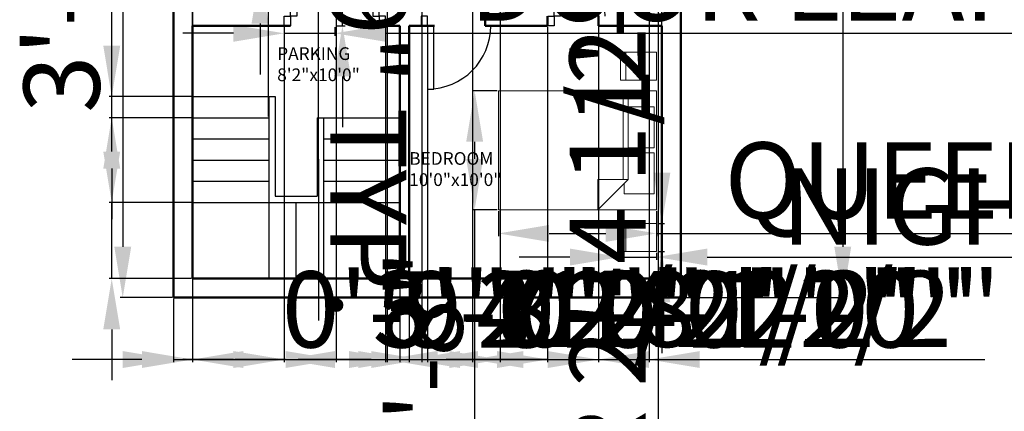
# Model space of a CAD drawing. Units: inches. Extents: x 1102 to 2414, y 295 to 1561.
# Tile 3 of 11: x 1505 to 1971, y 583 to 768. Entities that reach past the tile are written whole.
import ezdxf

# ---------------------------------------------------------------- set-up
doc = ezdxf.new("R2010")
doc.units = ezdxf.units.IN
for name, color, linetype, lineweight in [('A-ANNO-DIMS', 2, 'Continuous', 18), ('A-AREA-IDEN', 7, 'Continuous', 25), ('A-DOOR', 4, 'Continuous', 25), ('A-FLOR-STRS', 7, 'Continuous', 25), ('A-FURN', 8, 'Continuous', 18), ('A-WALL', 7, 'Continuous', 50)]:
    doc.layers.add(name, color=color, linetype=linetype, lineweight=lineweight)
doc.styles.get("Standard").update_dxf_attribs({"font": 'arial.ttf'})
doc.dimstyles.new('ISO-25', dxfattribs={"dimtxt": 36, "dimasz": 24, "dimexe": 1.25, "dimexo": 0.625, "dimtad": 1, "dimlunit": 4, "dimtxsty": 'Standard', "dimcen": 2.5, "dimadec": 0, "dimazin": 0, "dimtfac": 1, "dimtmove": 0, "dimatfit": 3, "dimfxl": 1, "dimarcsym": 0})

# ---------------------------------------------------------------- blocks, each defined once
blk = doc.blocks.new('*D2')
at = {"layer": 'A-ANNO-DIMS', "color": 0, "lineweight": -2, "transparency": 16777216}
for p, q in [((1576.92, 1116.76), (1552.25, 1116.76)), ((1553.5, 1092.76), (1553.5, 660.76)), ((1576.92, 636.76), (1552.25, 636.76))]:
    blk.add_line(p, q, dxfattribs=at)
at = {"layer": 'A-ANNO-DIMS', "color": 0, "transparency": 16777216}
for points in [[(1549.5, 1092.76), (1557.5, 1092.76), (1553.5, 1116.76)], [(1549.5, 660.76), (1557.5, 660.76), (1553.5, 636.76)]]:
    blk.add_solid(points, dxfattribs=at)
at = {"layer": 'Defpoints', "color": 0, "transparency": 16777216}
for p in [(1577.54, 1116.76), (1553.5, 636.76), (1577.54, 636.76)]:
    blk.add_point(p, dxfattribs=at)
at = {"layer": 'A-ANNO-DIMS', "color": 0, "transparency": 16777216, "insert": (1534.49, 876.76), "char_height": 36, "attachment_point": 5, "rotation": 90}
blk.add_mtext("40'", dxfattribs=at)
blk = doc.blocks.new('*D3')
at = {"layer": 'A-ANNO-DIMS', "color": 0, "lineweight": -2, "transparency": 16777216}
for p, q in [((1818.17, 1116.76), (1895.42, 1116.76)), ((1894.17, 1092.76), (1894.17, 660.76)), ((1818.17, 636.76), (1895.42, 636.76))]:
    blk.add_line(p, q, dxfattribs=at)
at = {"layer": 'A-ANNO-DIMS', "color": 0, "transparency": 16777216}
for points in [[(1890.17, 1092.76), (1898.17, 1092.76), (1894.17, 1116.76)], [(1890.17, 660.76), (1898.17, 660.76), (1894.17, 636.76)]]:
    blk.add_solid(points, dxfattribs=at)
at = {"layer": 'Defpoints', "color": 0, "transparency": 16777216}
for p in [(1817.54, 1116.76), (1817.54, 636.76), (1894.17, 636.76)]:
    blk.add_point(p, dxfattribs=at)
at = {"layer": 'A-ANNO-DIMS', "color": 0, "transparency": 16777216, "insert": (1875.16, 876.76), "char_height": 36, "attachment_point": 5, "rotation": 90}
blk.add_mtext("40'", dxfattribs=at)
blk = doc.blocks.new('Bed - Queen')
for p, q in [((0, -80.00003), (0, 0)), ((0, 0), (59.99999, 0)), ((59.99999, 0), (59.99999, -80.00003)), ((7.99999, -1.2), (28.79998, -1.2)), ((7.99999, -14.4), (7.99999, -1.2)), ((28.79998, -1.2), (28.79998, -14.4)), ((31.19999, -1.2), (51.99999, -1.2)), ((31.19999, -14.4), (31.19999, -1.2)), ((51.99999, -1.2), (51.99999, -16.4)), ((0, -14.4), (44.8, -14.4)), ((59.99999, -29.6), (44.8, -14.4)), ((44.8, -14.4), (44.8, -29.6)), ((44.8, -16.8), (0, -16.8)), ((51.99999, -16.4), (46.79936, -16.4)), ((44.8, -29.6), (59.99999, -29.6)), ((59.99999, -80.00003), (0, -80.00003))]:
    blk.add_line(p, q)
blk = doc.blocks.new('roomdoor')
for points in [[(1837.54, 1413.02), (1840.54, 1413.02), (1840.54, 1443.02), (1837.54, 1443.02)], [(1840.54, 1408.52), (1843.54, 1408.52), (1843.54, 1413.02), (1840.54, 1413.02)]]:
    blk.add_lwpolyline(points, close=True)
blk.add_arc((1840.54, 1413.02), 30, 90, 180)
blk = doc.blocks.new('utilitydoor')
for points in [[(1891.43, 1413.69), (1894.43, 1413.69), (1894.43, 1437.69), (1891.43, 1437.69)], [(1894.43, 1409.19), (1897.43, 1409.19), (1897.43, 1413.69), (1894.43, 1413.69)]]:
    blk.add_lwpolyline(points, close=True)
blk.add_arc((1894.43, 1413.69), 24, 90, 180)
blk = doc.blocks.new('TABLE-BEDSIDE')
for p, q in [((16.99, 13.29), (0, 13.29)), ((0, 13.29), (0, 0)), ((2.56, 0), (2.56, 13.29)), ((16.99, 0), (16.99, 13.29)), ((0, 0), (16.99, 0))]:
    blk.add_line(p, q)
blk = doc.blocks.new('DOOR-DOUBLE-LEAF-18')
blk.add_lwpolyline([(3, 22.5), (6, 22.5), (6, 4.5), (3, 4.5)], close=True)
blk.add_lwpolyline([(0, 0), (0, 4.5), (3, 4.5), (3, 0)])
blk.add_arc((6, 4.5), 18, 0, 90)
blk = doc.blocks.new('*D18')
at = {"layer": 'A-ANNO-DIMS', "color": 0, "lineweight": -2, "transparency": 16777216}
for p, q in [((1646.02, 927.81), (1646.02, 951.81)), ((1643.89, 903.81), (1647.27, 903.81)), ((1646.02, 903.81), (1646.02, 894.61)), ((1643.89, 894.6), (1647.27, 894.61)), ((1646.03, 870.61), (1646.05, 625.92))]:
    blk.add_line(p, q, dxfattribs=at)
at = {"layer": 'A-ANNO-DIMS', "color": 0, "transparency": 16777216}
for points in [[(1650.02, 927.81), (1642.02, 927.81), (1646.02, 903.81)], [(1650.03, 870.61), (1642.03, 870.6), (1646.02, 894.61)]]:
    blk.add_solid(points, dxfattribs=at)
at = {"layer": 'Defpoints', "color": 0, "transparency": 16777216}
for p in [(1643.27, 903.81), (1643.27, 894.6), (1646.02, 894.61)]:
    blk.add_point(p, dxfattribs=at)
at = {"layer": 'A-ANNO-DIMS', "color": 0, "transparency": 16777216, "insert": (1665.05, 736.26), "char_height": 36, "attachment_point": 5, "rotation": 270.0057}
blk.add_mtext('0\'-9" TYP.', dxfattribs=at)
blk = doc.blocks.new('*D19')
at = {"layer": 'A-ANNO-DIMS', "color": 0, "lineweight": -2, "transparency": 16777216}
for p, q in [((1789.04, 657.86), (1789.04, 654.68)), ((1806.03, 657.86), (1806.03, 654.68)), ((1765.04, 655.93), (1741.04, 655.93)), ((1789.04, 655.93), (1806.03, 655.93)), ((1830.03, 655.93), (2413.84, 655.93))]:
    blk.add_line(p, q, dxfattribs=at)
at = {"layer": 'A-ANNO-DIMS', "color": 0, "transparency": 16777216}
for points in [[(1765.04, 659.93), (1765.04, 651.93), (1789.04, 655.93)], [(1830.03, 659.93), (1830.03, 651.93), (1806.03, 655.93)]]:
    blk.add_solid(points, dxfattribs=at)
at = {"layer": 'Defpoints', "color": 0, "transparency": 16777216}
for p in [(1789.04, 658.48), (1806.03, 658.48), (1806.03, 655.93)]:
    blk.add_point(p, dxfattribs=at)
at = {"layer": 'A-ANNO-DIMS', "color": 0, "transparency": 16777216, "insert": (2133.94, 675.17), "char_height": 36, "attachment_point": 5}
blk.add_mtext('NIGHTSTAND 1\'-5" TYP.', dxfattribs=at)
blk = doc.blocks.new('*D20')
at = {"layer": 'A-ANNO-DIMS', "color": 0, "lineweight": -2, "transparency": 16777216}
for p, q in [((1808.58, 695.77), (1808.58, 1020.95)), ((1806.65, 671.77), (1809.83, 671.77)), ((1808.58, 658.48), (1808.58, 671.77)), ((1806.65, 658.48), (1809.83, 658.48)), ((1808.58, 634.48), (1808.58, 610.48))]:
    blk.add_line(p, q, dxfattribs=at)
at = {"layer": 'A-ANNO-DIMS', "color": 0, "transparency": 16777216}
for points in [[(1804.58, 695.77), (1812.58, 695.77), (1808.58, 671.77)], [(1804.58, 634.48), (1812.58, 634.48), (1808.58, 658.48)]]:
    blk.add_solid(points, dxfattribs=at)
at = {"layer": 'Defpoints', "color": 0, "transparency": 16777216}
for p in [(1806.03, 671.77), (1808.58, 671.77), (1806.03, 658.48)]:
    blk.add_point(p, dxfattribs=at)
at = {"layer": 'A-ANNO-DIMS', "color": 0, "transparency": 16777216, "insert": (1789.34, 870.36), "char_height": 36, "attachment_point": 5, "rotation": 90}
blk.add_mtext('1\'-1 1/2" TYP.', dxfattribs=at)
blk = doc.blocks.new('*D21')
at = {"layer": 'A-ANNO-DIMS', "color": 0, "lineweight": -2, "transparency": 16777216}
for p, q in [((1731.22, 677.69), (1731.22, 665.84)), ((1806.03, 677.69), (1806.03, 665.84)), ((1755.22, 667.09), (1782.03, 667.09)), ((1806.03, 667.09), (2237.1, 667.09))]:
    blk.add_line(p, q, dxfattribs=at)
at = {"layer": 'A-ANNO-DIMS', "color": 0, "transparency": 16777216}
for points in [[(1755.22, 671.09), (1755.22, 663.09), (1731.22, 667.09)], [(1782.03, 671.09), (1782.03, 663.09), (1806.03, 667.09)]]:
    blk.add_solid(points, dxfattribs=at)
at = {"layer": 'Defpoints', "color": 0, "transparency": 16777216}
for p in [(1731.22, 678.32), (1806.03, 678.32), (1806.03, 667.09)]:
    blk.add_point(p, dxfattribs=at)
at = {"layer": 'A-ANNO-DIMS', "color": 0, "transparency": 16777216, "insert": (2033.56, 687.44), "char_height": 36, "attachment_point": 5}
blk.add_mtext('QUEEN BED 6\'-3"', dxfattribs=at)
blk = doc.blocks.new('*D22')
at = {"layer": 'A-ANNO-DIMS', "color": 0, "lineweight": -2, "transparency": 16777216}
for p, q in [((1730.6, 734.42), (1718.75, 734.42)), ((1720, 710.42), (1720, 702.32)), ((1730.6, 678.32), (1718.75, 678.32)), ((1720, 678.32), (1720, 555.92))]:
    blk.add_line(p, q, dxfattribs=at)
at = {"layer": 'A-ANNO-DIMS', "color": 0, "transparency": 16777216}
for points in [[(1716, 710.42), (1724, 710.42), (1720, 734.42)], [(1716, 702.32), (1724, 702.32), (1720, 678.32)]]:
    blk.add_solid(points, dxfattribs=at)
at = {"layer": 'Defpoints', "color": 0, "transparency": 16777216}
for p in [(1731.22, 734.42), (1720, 678.32), (1731.22, 678.32)]:
    blk.add_point(p, dxfattribs=at)
at = {"layer": 'A-ANNO-DIMS', "color": 0, "transparency": 16777216, "insert": (1701, 605.12), "char_height": 36, "attachment_point": 5, "rotation": 90}
blk.add_mtext('4\'-8"', dxfattribs=at)
blk = doc.blocks.new('*D29')
at = {"layer": 'A-ANNO-DIMS', "color": 0, "lineweight": -2, "transparency": 16777216}
for p, q in [((1806.82, 1011.76), (1806.82, 1035.76)), ((1803.17, 987.76), (1808.07, 987.76)), ((1806.82, 987.76), (1806.82, 959.26)), ((1803.17, 959.26), (1808.07, 959.26)), ((1806.82, 935.26), (1806.82, 295.33))]:
    blk.add_line(p, q, dxfattribs=at)
at = {"layer": 'A-ANNO-DIMS', "color": 0, "transparency": 16777216}
for points in [[(1802.82, 1011.76), (1810.82, 1011.76), (1806.82, 987.76)], [(1802.82, 935.26), (1810.82, 935.26), (1806.82, 959.26)]]:
    blk.add_solid(points, dxfattribs=at)
at = {"layer": 'Defpoints', "color": 0, "transparency": 16777216}
for p in [(1802.54, 987.76), (1802.54, 959.26), (1806.82, 959.26)]:
    blk.add_point(p, dxfattribs=at)
at = {"layer": 'A-ANNO-DIMS', "color": 0, "transparency": 16777216, "insert": (1787.57, 603.3), "char_height": 36, "attachment_point": 5, "rotation": 90}
blk.add_mtext('BATH DOOR 2\'-4 1/2" TYP.', dxfattribs=at)
blk = doc.blocks.new('*D31')
at = {"layer": 'A-ANNO-DIMS', "color": 0, "lineweight": -2, "transparency": 16777216}
for p, q in [((1629.86, 764.63), (1629.86, 760.41)), ((1653.86, 764.63), (1653.86, 760.41)), ((1605.86, 761.66), (1581.86, 761.66)), ((1629.86, 761.66), (1653.86, 761.66)), ((1677.86, 761.66), (2225.36, 761.66))]:
    blk.add_line(p, q, dxfattribs=at)
at = {"layer": 'A-ANNO-DIMS', "color": 0, "transparency": 16777216}
for points in [[(1605.86, 765.66), (1605.86, 757.66), (1629.86, 761.66)], [(1677.86, 765.66), (1677.86, 757.66), (1653.86, 761.66)]]:
    blk.add_solid(points, dxfattribs=at)
at = {"layer": 'Defpoints', "color": 0, "transparency": 16777216}
for p in [(1629.86, 765.26), (1653.86, 765.26), (1653.86, 761.66)]:
    blk.add_point(p, dxfattribs=at)
at = {"layer": 'A-ANNO-DIMS', "color": 0, "transparency": 16777216, "insert": (1963.61, 780.91), "char_height": 36, "attachment_point": 5}
blk.add_mtext('DOOR LEAF 2\'-0" TYP.', dxfattribs=at)
blk = doc.blocks.new('*D32')
at = {"layer": 'A-ANNO-DIMS', "color": 0, "lineweight": -2, "transparency": 16777216}
for p, q in [((1657.46, 811.76), (1657.46, 1164.91)), ((1654.49, 787.76), (1658.71, 787.76)), ((1657.46, 765.26), (1657.46, 787.76)), ((1654.49, 765.26), (1658.71, 765.26)), ((1657.46, 741.26), (1657.46, 717.26))]:
    blk.add_line(p, q, dxfattribs=at)
at = {"layer": 'A-ANNO-DIMS', "color": 0, "transparency": 16777216}
for points in [[(1653.46, 811.76), (1661.46, 811.76), (1657.46, 787.76)], [(1653.46, 741.26), (1661.46, 741.26), (1657.46, 765.26)]]:
    blk.add_solid(points, dxfattribs=at)
at = {"layer": 'Defpoints', "color": 0, "transparency": 16777216}
for p in [(1653.86, 787.76), (1657.46, 787.76), (1653.86, 765.26)]:
    blk.add_point(p, dxfattribs=at)
at = {"layer": 'A-ANNO-DIMS', "color": 0, "transparency": 16777216, "insert": (1638.22, 1000.34), "char_height": 36, "attachment_point": 5, "rotation": 90}
blk.add_mtext('1\'-10 1/2" TYP.', dxfattribs=at)
blk = doc.blocks.new('*D37')
at = {"layer": 'A-ANNO-DIMS', "color": 0, "lineweight": -2, "transparency": 16777216}
for p, q in [((1618.46, 855.15), (1618.46, 1126.82)), ((1612.94, 831.15), (1619.71, 831.15)), ((1618.46, 790.23), (1618.46, 831.15)), ((1612.94, 790.23), (1619.71, 790.23)), ((1618.46, 766.23), (1618.46, 742.23))]:
    blk.add_line(p, q, dxfattribs=at)
at = {"layer": 'A-ANNO-DIMS', "color": 0, "transparency": 16777216}
for points in [[(1614.46, 855.15), (1622.46, 855.15), (1618.46, 831.15)], [(1614.46, 766.23), (1622.46, 766.23), (1618.46, 790.23)]]:
    blk.add_solid(points, dxfattribs=at)
at = {"layer": 'Defpoints', "color": 0, "transparency": 16777216}
for p in [(1612.32, 831.15), (1618.46, 831.15), (1612.32, 790.23)]:
    blk.add_point(p, dxfattribs=at)
at = {"layer": 'A-ANNO-DIMS', "color": 0, "transparency": 16777216, "insert": (1599.19, 1002.98), "char_height": 36, "attachment_point": 5, "rotation": 90}
blk.add_mtext('SOFA 3\'-5"', dxfattribs=at)
blk = doc.blocks.new('*D41')
at = {"layer": 'A-ANNO-DIMS', "color": 0, "lineweight": -2, "transparency": 16777216}
for p, q in [((1586.54, 645.13), (1586.54, 606.26)), ((1577.54, 636.13), (1577.54, 606.26)), ((1553.54, 607.51), (1529.54, 607.51)), ((1577.54, 607.51), (1586.54, 607.51)), ((1610.54, 607.51), (1731.49, 607.51))]:
    blk.add_line(p, q, dxfattribs=at)
at = {"layer": 'A-ANNO-DIMS', "color": 0, "transparency": 16777216}
for points in [[(1553.54, 611.51), (1553.54, 603.51), (1577.54, 607.51)], [(1610.54, 611.51), (1610.54, 603.51), (1586.54, 607.51)]]:
    blk.add_solid(points, dxfattribs=at)
at = {"layer": 'Defpoints', "color": 0, "transparency": 16777216}
for p in [(1586.54, 645.76), (1577.54, 636.76), (1586.54, 607.51)]:
    blk.add_point(p, dxfattribs=at)
at = {"layer": 'A-ANNO-DIMS', "color": 0, "transparency": 16777216, "insert": (1683.02, 626.52), "char_height": 36, "attachment_point": 5}
blk.add_mtext('0\'-9"', dxfattribs=at)
blk = doc.blocks.new('*D42')
at = {"layer": 'A-ANNO-DIMS', "color": 0, "lineweight": -2, "transparency": 16777216}
for p, q in [((1684.54, 645.13), (1684.54, 606.26)), ((1689.04, 645.13), (1689.04, 606.26)), ((1660.54, 607.51), (1636.54, 607.51)), ((1684.54, 607.51), (1689.04, 607.51)), ((1713.04, 607.51), (1917.88, 607.51))]:
    blk.add_line(p, q, dxfattribs=at)
at = {"layer": 'A-ANNO-DIMS', "color": 0, "transparency": 16777216}
for points in [[(1660.54, 611.51), (1660.54, 603.51), (1684.54, 607.51)], [(1713.04, 611.51), (1713.04, 603.51), (1689.04, 607.51)]]:
    blk.add_solid(points, dxfattribs=at)
at = {"layer": 'Defpoints', "color": 0, "transparency": 16777216}
for p in [(1684.54, 645.76), (1689.04, 645.76), (1689.04, 607.51)]:
    blk.add_point(p, dxfattribs=at)
at = {"layer": 'A-ANNO-DIMS', "color": 0, "transparency": 16777216, "insert": (1827.46, 626.75), "char_height": 36, "attachment_point": 5}
blk.add_mtext('0\'-4 1/2"', dxfattribs=at)
blk = doc.blocks.new('*D43')
at = {"layer": 'A-ANNO-DIMS', "color": 0, "lineweight": -2, "transparency": 16777216}
for p, q in [((1586.54, 764.63), (1586.54, 606.26)), ((1629.86, 764.63), (1629.86, 606.26)), ((1562.54, 607.51), (1538.54, 607.51)), ((1586.54, 607.51), (1629.86, 607.51)), ((1653.86, 607.51), (1858.67, 607.51))]:
    blk.add_line(p, q, dxfattribs=at)
at = {"layer": 'A-ANNO-DIMS', "color": 0, "transparency": 16777216}
for points in [[(1562.54, 611.51), (1562.54, 603.51), (1586.54, 607.51)], [(1653.86, 611.51), (1653.86, 603.51), (1629.86, 607.51)]]:
    blk.add_solid(points, dxfattribs=at)
at = {"layer": 'Defpoints', "color": 0, "transparency": 16777216}
for p in [(1586.54, 765.26), (1629.86, 765.26), (1629.86, 607.51)]:
    blk.add_point(p, dxfattribs=at)
at = {"layer": 'A-ANNO-DIMS', "color": 0, "transparency": 16777216, "insert": (1768.27, 626.76), "char_height": 36, "attachment_point": 5}
blk.add_mtext('3\'-7 1/2"', dxfattribs=at)
blk = doc.blocks.new('*D44')
at = {"layer": 'A-ANNO-DIMS', "color": 0, "lineweight": -2, "transparency": 16777216}
for p, q in [((1689.04, 764.63), (1689.04, 606.26)), ((1697.64, 764.63), (1697.64, 606.26)), ((1665.04, 607.51), (1641.04, 607.51)), ((1689.04, 607.51), (1697.64, 607.51)), ((1721.64, 607.51), (1926.48, 607.51))]:
    blk.add_line(p, q, dxfattribs=at)
at = {"layer": 'A-ANNO-DIMS', "color": 0, "transparency": 16777216}
for points in [[(1665.04, 611.51), (1665.04, 603.51), (1689.04, 607.51)], [(1721.64, 611.51), (1721.64, 603.51), (1697.64, 607.51)]]:
    blk.add_solid(points, dxfattribs=at)
at = {"layer": 'Defpoints', "color": 0, "transparency": 16777216}
for p in [(1689.04, 765.26), (1697.64, 765.26), (1697.64, 607.51)]:
    blk.add_point(p, dxfattribs=at)
at = {"layer": 'A-ANNO-DIMS', "color": 0, "transparency": 16777216, "insert": (1836.06, 626.75), "char_height": 36, "attachment_point": 5}
blk.add_mtext('0\'-8 1/2"', dxfattribs=at)
blk = doc.blocks.new('*D46')
at = {"layer": 'A-ANNO-DIMS', "color": 0, "lineweight": -2, "transparency": 16777216}
for p, q in [((1732.04, 857.63), (1732.04, 606.26)), ((1586.54, 853.13), (1586.54, 606.26)), ((1610.54, 607.51), (1708.04, 607.51)), ((1732.04, 607.51), (1961.46, 607.51))]:
    blk.add_line(p, q, dxfattribs=at)
at = {"layer": 'A-ANNO-DIMS', "color": 0, "transparency": 16777216}
for points in [[(1610.54, 611.51), (1610.54, 603.51), (1586.54, 607.51)], [(1708.04, 611.51), (1708.04, 603.51), (1732.04, 607.51)]]:
    blk.add_solid(points, dxfattribs=at)
at = {"layer": 'Defpoints', "color": 0, "transparency": 16777216}
for p in [(1732.04, 858.26), (1586.54, 853.76), (1732.04, 607.51)]:
    blk.add_point(p, dxfattribs=at)
at = {"layer": 'A-ANNO-DIMS', "color": 0, "transparency": 16777216, "insert": (1858.75, 626.75), "char_height": 36, "attachment_point": 5}
blk.add_mtext('12\'-1 1/2"', dxfattribs=at)
blk = doc.blocks.new('*D50')
at = {"layer": 'A-ANNO-DIMS', "color": 0, "lineweight": -2, "transparency": 16777216}
for p, q in [((1586.54, 987.13), (1586.54, 606.26)), ((1654.54, 987.13), (1654.54, 606.26)), ((1610.54, 607.51), (1630.54, 607.51)), ((1654.54, 607.51), (1775.49, 607.51))]:
    blk.add_line(p, q, dxfattribs=at)
at = {"layer": 'A-ANNO-DIMS', "color": 0, "transparency": 16777216}
for points in [[(1610.54, 611.51), (1610.54, 603.51), (1586.54, 607.51)], [(1630.54, 611.51), (1630.54, 603.51), (1654.54, 607.51)]]:
    blk.add_solid(points, dxfattribs=at)
at = {"layer": 'Defpoints', "color": 0, "transparency": 16777216}
for p in [(1586.54, 987.76), (1654.54, 987.76), (1654.54, 607.51)]:
    blk.add_point(p, dxfattribs=at)
at = {"layer": 'A-ANNO-DIMS', "color": 0, "transparency": 16777216, "insert": (1727.02, 626.52), "char_height": 36, "attachment_point": 5}
blk.add_mtext('5\'-8"', dxfattribs=at)
blk = doc.blocks.new('*D55')
at = {"layer": 'A-ANNO-DIMS', "color": 0, "lineweight": -2, "transparency": 16777216}
for p, q in [((1562.54, 1146.01), (1538.54, 1146.01)), ((1586.54, 722.38), (1586.54, 1147.26)), ((1586.54, 1146.01), (1622.54, 1146.01)), ((1622.54, 722.38), (1622.54, 1147.26)), ((1646.54, 1146.01), (1767.47, 1146.01))]:
    blk.add_line(p, q, dxfattribs=at)
at = {"layer": 'A-ANNO-DIMS', "color": 0, "transparency": 16777216}
for points in [[(1562.54, 1150.01), (1562.54, 1142.01), (1586.54, 1146.01)], [(1646.54, 1150.01), (1646.54, 1142.01), (1622.54, 1146.01)]]:
    blk.add_solid(points, dxfattribs=at)
at = {"layer": 'Defpoints', "color": 0, "transparency": 16777216}
for p in [(1622.54, 1146.01), (1586.54, 721.76), (1622.54, 721.76)]:
    blk.add_point(p, dxfattribs=at)
at = {"layer": 'A-ANNO-DIMS', "color": 0, "transparency": 16777216, "insert": (1719.01, 1165.03), "char_height": 36, "attachment_point": 5}
blk.add_mtext('3\'-0"', dxfattribs=at)
blk = doc.blocks.new('*D56')
at = {"layer": 'A-ANNO-DIMS', "color": 0, "lineweight": -2, "transparency": 16777216}
for p, q in [((1548.29, 705.76), (1548.29, 826.68)), ((1585.92, 681.76), (1547.04, 681.76)), ((1548.29, 645.76), (1548.29, 681.76)), ((1585.92, 645.76), (1547.04, 645.76)), ((1548.29, 621.76), (1548.29, 597.76))]:
    blk.add_line(p, q, dxfattribs=at)
at = {"layer": 'A-ANNO-DIMS', "color": 0, "transparency": 16777216}
for points in [[(1544.29, 705.76), (1552.29, 705.76), (1548.29, 681.76)], [(1544.29, 621.76), (1552.29, 621.76), (1548.29, 645.76)]]:
    blk.add_solid(points, dxfattribs=at)
at = {"layer": 'Defpoints', "color": 0, "transparency": 16777216}
for p in [(1548.29, 681.76), (1586.54, 681.76), (1586.54, 645.76)]:
    blk.add_point(p, dxfattribs=at)
at = {"layer": 'A-ANNO-DIMS', "color": 0, "transparency": 16777216, "insert": (1529.28, 778.22), "char_height": 36, "attachment_point": 5, "rotation": 90}
blk.add_mtext('3\'-0"', dxfattribs=at)
blk = doc.blocks.new('*D57')
at = {"layer": 'A-ANNO-DIMS', "color": 0, "lineweight": -2, "transparency": 16777216}
for p, q in [((1548.29, 755.76), (1548.29, 904.68)), ((1585.92, 731.76), (1547.04, 731.76)), ((1548.29, 721.76), (1548.29, 731.76)), ((1585.92, 721.76), (1547.04, 721.76)), ((1548.29, 697.76), (1548.29, 673.76))]:
    blk.add_line(p, q, dxfattribs=at)
at = {"layer": 'A-ANNO-DIMS', "color": 0, "transparency": 16777216}
for points in [[(1544.29, 755.76), (1552.29, 755.76), (1548.29, 731.76)], [(1544.29, 697.76), (1552.29, 697.76), (1548.29, 721.76)]]:
    blk.add_solid(points, dxfattribs=at)
at = {"layer": 'Defpoints', "color": 0, "transparency": 16777216}
for p in [(1548.29, 731.76), (1586.54, 731.76), (1586.54, 721.76)]:
    blk.add_point(p, dxfattribs=at)
at = {"layer": 'A-ANNO-DIMS', "color": 0, "transparency": 16777216, "insert": (1529.29, 842.22), "char_height": 36, "attachment_point": 5, "rotation": 90}
blk.add_mtext('0\'-10"', dxfattribs=at)
blk = doc.blocks.new('*D62')
at = {"layer": 'A-ANNO-DIMS', "color": 0, "lineweight": -2, "transparency": 16777216}
for p, q in [((1778.54, 982.63), (1778.54, 606.26)), ((1802.54, 982.63), (1802.54, 606.26)), ((1754.54, 607.51), (1730.54, 607.51)), ((1778.54, 607.51), (1802.54, 607.51)), ((1826.54, 607.51), (1948.11, 607.51))]:
    blk.add_line(p, q, dxfattribs=at)
at = {"layer": 'A-ANNO-DIMS', "color": 0, "transparency": 16777216}
for points in [[(1754.54, 611.51), (1754.54, 603.51), (1778.54, 607.51)], [(1826.54, 611.51), (1826.54, 603.51), (1802.54, 607.51)]]:
    blk.add_solid(points, dxfattribs=at)
at = {"layer": 'Defpoints', "color": 0, "transparency": 16777216}
for p in [(1778.54, 983.26), (1802.54, 983.26), (1802.54, 607.51)]:
    blk.add_point(p, dxfattribs=at)
at = {"layer": 'A-ANNO-DIMS', "color": 0, "transparency": 16777216, "insert": (1899.32, 626.52), "char_height": 36, "attachment_point": 5}
blk.add_mtext('2\'-0"', dxfattribs=at)
blk = doc.blocks.new('*D63')
at = {"layer": 'A-ANNO-DIMS', "color": 0, "lineweight": -2, "transparency": 16777216}
for p, q in [((1654.54, 982.63), (1654.54, 606.26)), ((1678.54, 982.63), (1678.54, 606.26)), ((1630.54, 607.51), (1606.54, 607.51)), ((1654.54, 607.51), (1678.54, 607.51)), ((1702.54, 607.51), (1824.11, 607.51))]:
    blk.add_line(p, q, dxfattribs=at)
at = {"layer": 'A-ANNO-DIMS', "color": 0, "transparency": 16777216}
for points in [[(1630.54, 611.51), (1630.54, 603.51), (1654.54, 607.51)], [(1702.54, 611.51), (1702.54, 603.51), (1678.54, 607.51)]]:
    blk.add_solid(points, dxfattribs=at)
at = {"layer": 'Defpoints', "color": 0, "transparency": 16777216}
for p in [(1654.54, 983.26), (1678.54, 983.26), (1678.54, 607.51)]:
    blk.add_point(p, dxfattribs=at)
at = {"layer": 'A-ANNO-DIMS', "color": 0, "transparency": 16777216, "insert": (1775.32, 626.52), "char_height": 36, "attachment_point": 5}
blk.add_mtext('2\'-0"', dxfattribs=at)
blk = doc.blocks.new('*D64')
at = {"layer": 'A-ANNO-DIMS', "color": 0, "lineweight": -2, "transparency": 16777216}
for p, q in [((1695.04, 982.63), (1695.04, 606.26)), ((1719.04, 982.63), (1719.04, 606.26)), ((1671.04, 607.51), (1647.04, 607.51)), ((1695.04, 607.51), (1719.04, 607.51)), ((1743.04, 607.51), (1864.61, 607.51))]:
    blk.add_line(p, q, dxfattribs=at)
at = {"layer": 'A-ANNO-DIMS', "color": 0, "transparency": 16777216}
for points in [[(1671.04, 611.51), (1671.04, 603.51), (1695.04, 607.51)], [(1743.04, 611.51), (1743.04, 603.51), (1719.04, 607.51)]]:
    blk.add_solid(points, dxfattribs=at)
at = {"layer": 'Defpoints', "color": 0, "transparency": 16777216}
for p in [(1695.04, 983.26), (1719.04, 983.26), (1719.04, 607.51)]:
    blk.add_point(p, dxfattribs=at)
at = {"layer": 'A-ANNO-DIMS', "color": 0, "transparency": 16777216, "insert": (1815.82, 626.52), "char_height": 36, "attachment_point": 5}
blk.add_mtext('2\'-0"', dxfattribs=at)
blk = doc.blocks.new('*D66')
at = {"layer": 'A-ANNO-DIMS', "color": 0, "lineweight": -2, "transparency": 16777216}
for p, q in [((1629.86, 764.63), (1629.86, 606.26)), ((1677.86, 764.63), (1677.86, 606.26)), ((1605.86, 607.51), (1581.86, 607.51)), ((1629.86, 607.51), (1677.86, 607.51)), ((1701.86, 607.51), (1824.26, 607.51))]:
    blk.add_line(p, q, dxfattribs=at)
at = {"layer": 'A-ANNO-DIMS', "color": 0, "transparency": 16777216}
for points in [[(1605.86, 611.51), (1605.86, 603.51), (1629.86, 607.51)], [(1701.86, 611.51), (1701.86, 603.51), (1677.86, 607.51)]]:
    blk.add_solid(points, dxfattribs=at)
at = {"layer": 'Defpoints', "color": 0, "transparency": 16777216}
for p in [(1629.86, 765.26), (1677.86, 765.26), (1677.86, 607.51)]:
    blk.add_point(p, dxfattribs=at)
at = {"layer": 'A-ANNO-DIMS', "color": 0, "transparency": 16777216, "insert": (1775.06, 626.52), "char_height": 36, "attachment_point": 5}
blk.add_mtext('4\'-0"', dxfattribs=at)
blk = doc.blocks.new('*D67')
at = {"layer": 'A-ANNO-DIMS', "color": 0, "lineweight": -2, "transparency": 16777216}
for p, q in [((1754.54, 764.63), (1754.54, 606.26)), ((1778.54, 764.63), (1778.54, 606.26)), ((1730.54, 607.51), (1706.54, 607.51)), ((1754.54, 607.51), (1778.54, 607.51)), ((1802.54, 607.51), (1924.11, 607.51))]:
    blk.add_line(p, q, dxfattribs=at)
at = {"layer": 'A-ANNO-DIMS', "color": 0, "transparency": 16777216}
for points in [[(1730.54, 611.51), (1730.54, 603.51), (1754.54, 607.51)], [(1802.54, 611.51), (1802.54, 603.51), (1778.54, 607.51)]]:
    blk.add_solid(points, dxfattribs=at)
at = {"layer": 'Defpoints', "color": 0, "transparency": 16777216}
for p in [(1754.54, 765.26), (1778.54, 765.26), (1778.54, 607.51)]:
    blk.add_point(p, dxfattribs=at)
at = {"layer": 'A-ANNO-DIMS', "color": 0, "transparency": 16777216, "insert": (1875.32, 626.52), "char_height": 36, "attachment_point": 5}
blk.add_mtext('2\'-0"', dxfattribs=at)

msp = doc.modelspace()

# ---------------------------------------------------------------- linework, layer by layer
at = {"layer": 'A-FLOR-STRS'}
for p, q in [((1586.544, 731.76), (1625.544, 731.76)), ((1622.544, 731.76), (1622.544, 645.76)), ((1625.544, 731.76), (1625.544, 684.76)), ((1586.544, 721.76), (1622.544, 721.76)), ((1645.544, 721.76), (1645.544, 684.76)), ((1645.544, 721.76), (1684.544, 721.76)), ((1648.544, 721.76), (1648.544, 645.76)), ((1586.544, 711.76), (1622.544, 711.76)), ((1648.544, 711.76), (1684.544, 711.76)), ((1586.544, 701.76), (1622.544, 701.76)), ((1648.544, 701.76), (1684.544, 701.76)), ((1586.544, 691.76), (1622.544, 691.76)), ((1648.544, 691.76), (1684.544, 691.76)), ((1586.544, 681.76), (1684.544, 681.76)), ((1625.544, 684.76), (1645.544, 684.76)), ((1635.544, 645.76), (1635.544, 681.76))]:
    msp.add_line(p, q, dxfattribs=at)
at = {"layer": 'A-WALL'}
for p, q in [((1577.544, 1116.76), (1577.544, 636.76)), ((1817.544, 636.76), (1817.544, 1116.76)), ((1725.044, 769.76), (1725.044, 765.26)), ((1754.544, 769.76), (1754.544, 765.26)), ((1778.544, 769.76), (1778.544, 765.26)), ((1586.544, 765.26), (1586.544, 645.76)), ((1632.864, 765.26), (1586.544, 765.26)), ((1684.544, 765.26), (1674.864, 765.26)), ((1684.544, 765.26), (1684.544, 645.76)), ((1689.044, 765.26), (1689.044, 645.76)), ((1701.044, 765.26), (1689.044, 765.26)), ((1754.544, 765.26), (1725.044, 765.26)), ((1808.544, 765.26), (1778.544, 765.26)), ((1808.544, 645.76), (1808.544, 765.26)), ((1586.544, 645.76), (1684.544, 645.76)), ((1689.044, 645.76), (1808.544, 645.76)), ((1577.544, 636.76), (1817.544, 636.76))]:
    msp.add_line(p, q, dxfattribs=at)

# ---------------------------------------------------------------- block references
at = {"layer": 'A-DOOR', "xscale": -1}
msp.add_blockref('utilitydoor', (3651.978, -643.928), dxfattribs=at)
at = {"layer": 'A-DOOR'}
msp.add_blockref('DOOR-DOUBLE-LEAF-18', (1629.864, 765.26), dxfattribs=at)
at = {"layer": 'A-DOOR', "extrusion": (0, 0, -1), "zscale": -1}
msp.add_blockref('DOOR-DOUBLE-LEAF-18', (-1677.863, 765.26), dxfattribs=at)
at = {"layer": 'A-DOOR', "rotation": 180}
msp.add_blockref('roomdoor', (3538.188, 2178.278), dxfattribs=at)
at = {"layer": 'A-FURN'}
for p in [(1789.038, 739.454), (1789.038, 658.482)]:
    msp.add_blockref('TABLE-BEDSIDE', p, dxfattribs=at)
at = {"layer": 'A-FURN', "xscale": 0.9350450939157223, "yscale": 0.9350450939157223, "zscale": 0.9350450939157223, "rotation": 270}
msp.add_blockref('Bed - Queen', (1806.028, 734.418), dxfattribs=at)

# ---------------------------------------------------------------- texts
at = {"layer": 'A-AREA-IDEN', "char_height": 6, "attachment_point": 1}
for s, insert in [('PARKING\\P8\'2"x10\'0"', (1626.577, 755.048)), ('BEDROOM\\P10\'0"x10\'0"', (1689.044, 705.51))]:
    msp.add_mtext_dynamic_manual_height_columns(s, width=50.64919, gutter_width=12.5, heights=[0], dxfattribs=dict(at, insert=insert))

# ---------------------------------------------------------------- dimensions: what is measured, and where the dimension line sits
at = {"layer": 'A-ANNO-DIMS'}
for base, p1, p2, picture, middle in [((1622.544, 1146.01), (1586.544, 721.76), (1622.544, 721.76), '*D55', (1719.005, 1165.028)), ((1654.544, 607.51), (1586.544, 987.76), (1654.544, 987.76), '*D50', (1727.018, 626.515)), ((1678.544, 607.51), (1654.544, 983.26), (1678.544, 983.26), '*D63', (1775.325, 626.515)), ((1719.044, 607.51), (1695.044, 983.26), (1719.044, 983.26), '*D64', (1815.825, 626.515)), ((1802.544, 607.51), (1778.544, 983.26), (1802.544, 983.26), '*D62', (1899.325, 626.515)), ((1732.044, 607.51), (1586.544, 853.76), (1732.044, 858.26), '*D46', (1858.751, 626.749)), ((1629.864, 607.51), (1586.544, 765.26), (1629.864, 765.26), '*D43', (1768.268, 626.761)), ((1677.864, 607.51), (1629.864, 765.26), (1677.864, 765.26), '*D66', (1775.062, 626.515)), ((1697.644, 607.51), (1689.044, 765.26), (1697.644, 765.26), '*D44', (1836.06, 626.749)), ((1778.544, 607.51), (1754.544, 765.26), (1778.544, 765.26), '*D67', (1875.325, 626.515)), ((1689.044, 607.51), (1684.544, 645.76), (1689.044, 645.76), '*D42', (1827.46, 626.749)), ((1586.544, 607.51), (1577.544, 636.76), (1586.544, 645.76), '*D41', (1683.018, 626.515))]:
    dim = msp.add_linear_dim(base=base, p1=p1, p2=p2, dimstyle='ISO-25', override={"dimdec": 1, "dimlfac": 1, "dimrnd": 0, "dimzin": 1, "dimdsep": 46, "dimlunit": 4, "dimfrac": 2}, dxfattribs=at)
    dim.commit()
    dim.dimension.update_dxf_attribs({"geometry": picture, "text_midpoint": middle})
for base, p1, p2, angle, text, picture, middle in [((1657.464, 787.76), (1653.864, 765.26), (1653.864, 787.76), 90, '<> TYP.', '*D32', (1638.225, 1000.337)), ((1618.456, 831.145), (1612.319, 790.233), (1612.319, 831.145), 90, 'SOFA <>', '*D37', (1599.192, 1002.983)), ((1806.819, 959.26), (1802.544, 987.76), (1802.544, 959.26), 270, 'BATH DOOR <> TYP.', '*D29', (1787.568, 603.296)), ((1808.577, 671.77), (1806.028, 658.482), (1806.028, 671.77), 90, '<> TYP.', '*D20', (1789.338, 870.362)), ((1646.024, 894.605), (1643.268, 903.806), (1643.269, 894.605), 270.00567, '<> TYP.', '*D18', (1665.045, 736.263))]:
    dim = msp.add_linear_dim(base=base, p1=p1, p2=p2, angle=angle, text=text, dimstyle='ISO-25', override={"dimdec": 1, "dimlfac": 1, "dimrnd": 0, "dimzin": 1, "dimdsep": 46, "dimlunit": 4, "dimfrac": 2}, dxfattribs=at)
    dim.commit()
    dim.dimension.update_dxf_attribs({"geometry": picture, "text_midpoint": middle})
for base, p1, p2, angle, override, picture, middle in [((1553.496, 636.76), (1577.544, 1116.76), (1577.544, 636.76), 90, {"dimclrd": 0, "dimclre": 0, "dimclrt": 0}, '*D2', (1534.49, 876.76)), ((1548.294, 731.76), (1586.544, 721.76), (1586.544, 731.76), 90, {"dimdec": 1, "dimlfac": 1, "dimrnd": 0, "dimzin": 1, "dimdsep": 46, "dimlunit": 4, "dimfrac": 2}, '*D57', (1529.288, 842.218)), ((1548.294, 681.76), (1586.544, 645.76), (1586.544, 681.76), 90, {"dimdec": 1, "dimlfac": 1, "dimrnd": 0, "dimzin": 1, "dimdsep": 46, "dimlunit": 4, "dimfrac": 2}, '*D56', (1529.276, 778.221)), ((1720.004, 678.315), (1731.225, 734.418), (1731.225, 678.315), 270, {"dimdec": 1, "dimlfac": 1, "dimrnd": 0, "dimzin": 1, "dimdsep": 46, "dimlunit": 4, "dimfrac": 2}, '*D22', (1700.999, 605.118))]:
    dim = msp.add_linear_dim(base=base, p1=p1, p2=p2, angle=angle, dimstyle='ISO-25', override=override, dxfattribs=at)
    dim.commit()
    dim.dimension.update_dxf_attribs({"geometry": picture, "text_midpoint": middle})
dim = msp.add_linear_dim(base=(1894.167, 636.76), p1=(1817.544, 1116.76), p2=(1817.544, 636.76), angle=90, dimstyle='ISO-25', override={"dimclrd": 0, "dimclre": 0, "dimclrt": 0}, dxfattribs=at)
dim.commit()
dim.dimension.update_dxf_attribs({"geometry": '*D3', "text_midpoint": (1894.167, 876.76), "dimtype": 160})
for base, p1, p2, text, picture, middle in [((1653.864, 761.66), (1629.864, 765.26), (1653.864, 765.26), 'DOOR LEAF <> TYP.', '*D31', (1963.611, 780.911)), ((1806.028, 667.095), (1731.225, 678.315), (1806.028, 678.315), 'QUEEN BED <>', '*D21', (2033.565, 687.439)), ((1806.028, 655.933), (1789.038, 658.482), (1806.028, 658.482), 'NIGHTSTAND <> TYP.', '*D19', (2133.936, 675.172))]:
    dim = msp.add_linear_dim(base=base, p1=p1, p2=p2, text=text, dimstyle='ISO-25', override={"dimdec": 1, "dimlfac": 1, "dimrnd": 0, "dimzin": 1, "dimdsep": 46, "dimlunit": 4, "dimfrac": 2}, dxfattribs=at)
    dim.commit()
    dim.dimension.update_dxf_attribs({"geometry": picture, "text_midpoint": middle})

doc.saveas('drawing.dxf')
